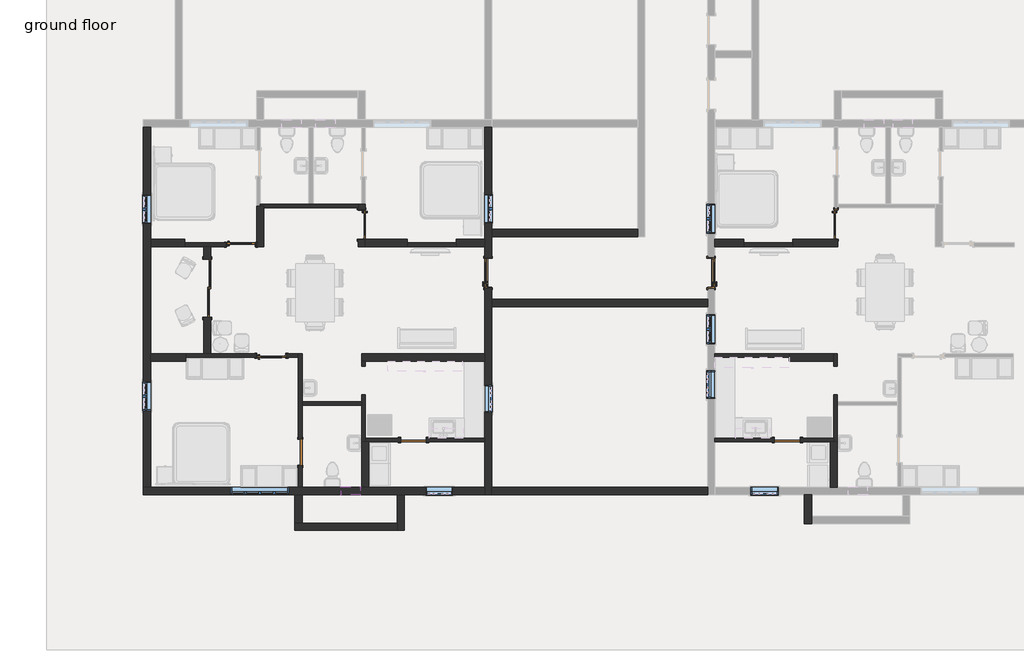
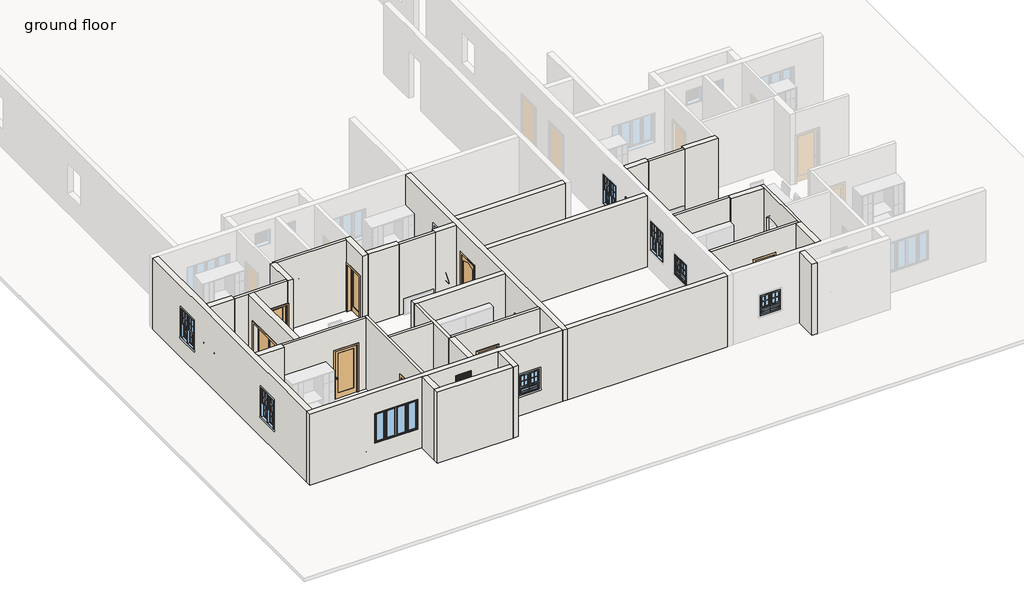
# One storey, part 1 of 16: 35 walls, 11 windows, 10 doors.
# Revit data of these elements (continued)
# Elements 4, 5, 6, 7 (IfcDoor, "Door-Interior-Single-1_Panel-Wood : 36\" x 84\"")
#   Swing Angle = 90.00°
#   Phase Created = New Construction
#   Materials on its faces: "Cherry", "Aluminum"
# Elements 8, 9, 10 (IfcDoor, "Single-Flush : 32\" x 84\"")
#   Phase Created = New Construction
#   Materials on its faces: "Door - Frame", "Door - Panel"
# Elements 11, 12, 13, 14, 15, 16, 17, 18, 19, 20, 21, 22 (IfcWall, "Generic - 4.5\"")
#   Top Offset = 0' - 0"
#   Base Offset = 0' - 0"
#   wall height = 10' - 6"
#   Phase Created = New Construction
#   Base Constraint = ground floor
#   Top Constraint = 1st floor
#   Materials on its faces: "Default Wall"
# Elements 23, 24, 25, 26, 27, 28, 29, 30, 31, 32, 33, 34, 35, 36, 37, 38, 39, 40, 41, 42, 43, 44, 45 (IfcWall, "Generic - 9\"")
#   Top Offset = 0' - 0"
#   Base Offset = 0' - 0"
#   wall height = 10' - 6"
#   Phase Created = New Construction
#   Base Constraint = ground floor
#   Top Constraint = 1st floor
#   Materials on its faces: "Default Wall"
# Element 46 (IfcWindow, "Window-Casement-Double-Awning : 34\" x 36\"")
#   Mark = "78"
#   Window Inset = 0' - 0"
#   Interior Wall Closure = 0' - 2 1/4"
#   Frame Extension = 0' - 0 1/4"
#   Exterior Wall Closure = 0' - 1 1/4"
#   Interior Trim Visibility = yes
#   Exterior Trim Visibility = yes
#   Phase Created = New Construction
#   Materials on its faces: "Wood - Stained", "Glass", "Clad - White"
# Element 47 (IfcWindow, "Window-Casement-Double-Awning : 34\" x 36\"")
#   Mark = "79"
#   Window Inset = 0' - 0"
#   Interior Wall Closure = 0' - 2 1/4"
#   Frame Extension = 0' - 0 1/4"
#   Exterior Wall Closure = 0' - 1 1/4"
#   Interior Trim Visibility = yes
#   Exterior Trim Visibility = yes
#   Phase Created = New Construction
#   Materials on its faces: "Wood - Stained", "Glass", "Clad - White"
# Element 48 (IfcWindow, "Window-Casement-Double-Awning : 34\" x 36\"")
#   Mark = "81"
#   Window Inset = 0' - 0"
#   Interior Wall Closure = 0' - 2 1/4"
#   Frame Extension = 0' - 0 1/4"
#   Exterior Wall Closure = 0' - 1 1/4"
#   Interior Trim Visibility = yes
#   Exterior Trim Visibility = yes
#   Phase Created = New Construction
#   Materials on its faces: "Wood - Stained", "Glass", "Clad - White"
# Element 49 (IfcWindow, "Window-Casement-Double-Awning : 34\" x 36\"")
#   Mark = "82"
#   Window Inset = 0' - 0"
#   Interior Wall Closure = 0' - 2 1/4"
#   Frame Extension = 0' - 0 1/4"
#   Exterior Wall Closure = 0' - 1 1/4"
#   Interior Trim Visibility = yes
#   Exterior Trim Visibility = yes
#   Phase Created = New Construction
#   Materials on its faces: "Wood - Stained", "Glass", "Clad - White"
# Element 50 (IfcWindow, "Window-Casement-Multi-Sash-Horizontal : 72\" x 53\"")
#   Mark = "31"
#   Window Inset = 0' - 0 5/8"
#   Frame Gap 3 = 0' - 1 83/128"
#   Frame Gap 2 = 0' - 0 5/8"
#   Phase Created = New Construction
#   Materials on its faces: "Metal - Aluminum", "Glass"
# Element 51 (IfcWindow, "Window-Louvers : 24\" x 24\"")
#   Mark = "103"
#   Blade Width = 1' - 10 1/2"
#   Phase Created = New Construction
#   Materials on its faces: "Birch"
# Element 52 (IfcWindow, "Window-Single-Hung-Double : 36\" x 52\"")
#   Mark = "54"
#   Window Inset = 0' - 0"
#   Interior Wall Closure = 0' - 1 1/2"
#   Frame Extension = 0' - 1 1/4"
#   Exterior Wall Closure = 0' - 0 1/2"
#   Interior Trim Visibility = yes
#   Indicator Visibility = yes
#   Exterior Trim Visibility = yes
#   Phase Created = New Construction
#   Materials on its faces: "Wood - Stained", "Glass", "Clad - White"
# Element 53 (IfcWindow, "Window-Single-Hung-Double : 36\" x 52\"")
#   Mark = "55"
#   Window Inset = 0' - 0"
#   Interior Wall Closure = 0' - 1 1/2"
#   Frame Extension = 0' - 1 1/4"
#   Exterior Wall Closure = 0' - 0 1/2"
#   Interior Trim Visibility = yes
#   Indicator Visibility = yes
#   Exterior Trim Visibility = yes
#   Phase Created = New Construction
#   Materials on its faces: "Wood - Stained", "Glass", "Clad - White"
# Element 54 (IfcWindow, "Window-Single-Hung-Double : 36\" x 52\"")
#   Mark = "56"
#   Window Inset = 0' - 0"
#   Interior Wall Closure = 0' - 1 1/2"
#   Frame Extension = 0' - 1 1/4"
#   Exterior Wall Closure = 0' - 0 1/2"
#   Interior Trim Visibility = yes
#   Indicator Visibility = yes
#   Exterior Trim Visibility = yes
#   Phase Created = New Construction
#   Materials on its faces: "Wood - Stained", "Glass", "Clad - White"
# Element 55 (IfcWindow, "Window-Single-Hung-Double : 36\" x 52\"")
#   Mark = "57"
#   Window Inset = 0' - 0"
#   Interior Wall Closure = 0' - 1 1/2"
#   Frame Extension = 0' - 1 1/4"
#   Exterior Wall Closure = 0' - 0 1/2"
#   Interior Trim Visibility = yes
#   Indicator Visibility = yes
#   Exterior Trim Visibility = yes
#   Phase Created = New Construction
#   Materials on its faces: "Wood - Stained", "Glass", "Clad - White"
# Element 56 (IfcWindow, "Window-Single-Hung-Double : 36\" x 52\"")
#   Mark = "80"
#   Window Inset = 0' - 0"
#   Interior Wall Closure = 0' - 1 1/2"
#   Frame Extension = 0' - 1 1/4"
#   Exterior Wall Closure = 0' - 0 1/2"
#   Interior Trim Visibility = yes
#   Indicator Visibility = yes
#   Exterior Trim Visibility = yes
#   Phase Created = New Construction
#   Materials on its faces: "Wood - Stained", "Glass", "Clad - White"
# Materials
#   "Cherry": class "Wood", colour RGB 226 177 128, transparency 0, Description = "Prunus Serotina", Cost = 0
#   "Glass": class "Glass", colour RGB 0 128 192, transparency 0.75, Description = "Soda Lime Glass", Cost = 0
#   "Aluminum": class "Metal", colour RGB 247 247 247, transparency 0, Description = "Aluminum 6061", Cost = 0
#   "Wood - Birch - Solid Stained Light Low Gloss": class "Wood", colour RGB 210 159 95, transparency 0, Cost = 0
#   "Paint - Sienna": colour RGB 118 70 51, transparency 0, Cost = 0
#   "Door - Panel": class "Wood", colour RGB 210 159 95, transparency 0, Cost = 0
#   "Door - Frame": colour RGB 118 70 51, transparency 0, Cost = 0
#   "Wood - Stained": class "Wood", colour RGB 224 178 126, transparency 0, Cost = 0
#   "Clad - White": class "Wood", colour RGB 242 242 238, transparency 0, Cost = 0
#   "Metal - Aluminum": class "Metal", colour RGB 247 247 247, transparency 0
#   "Birch": class "Wood", colour RGB 224 178 126, transparency 0, Description = "Betula Alleghaniensis", Cost = 0
#   "Default Wall": colour RGB 128 128 128, transparency 0, Cost = 0
